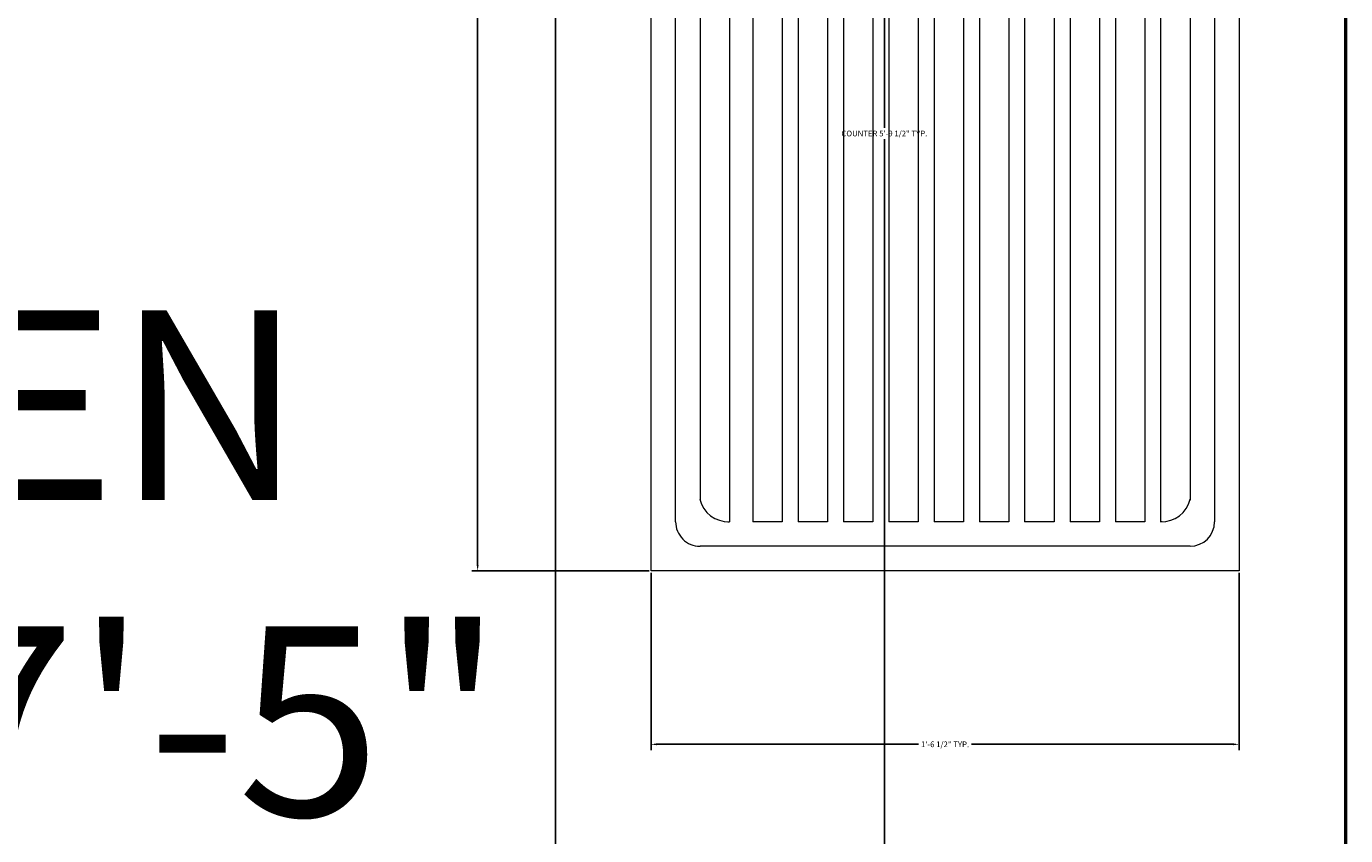
# Model space of a CAD drawing. Units: inches. Extents: x -173 to 545, y -746 to 104.
# Tile 27 of 32: x 219 to 261, y -69 to -43. Entities that reach past the tile are written whole.
import ezdxf

# ---------------------------------------------------------------- set-up
doc = ezdxf.new("R2010")
doc.units = ezdxf.units.IN
doc.header["$MEASUREMENT"] = 0
for name, color, linetype, lineweight in [('A-ANNO-DIMS', 2, 'Continuous', 18), ('A-AREA-IDEN', 7, 'Continuous', 18), ('A-FLOR-CASE', 9, 'Continuous', 25), ('A-FLOR-FIXT', 8, 'Continuous', 18), ('A-WALL', 7, 'Continuous', 50)]:
    doc.layers.add(name, color=color, linetype=linetype, lineweight=lineweight)
doc.styles.get("Standard").update_dxf_attribs({"font": 'arial.ttf'})
doc.dimstyles.get("Standard").update_dxf_attribs({"dimtxt": 0.18, "dimasz": 0.18, "dimexe": 0.18, "dimexo": 0.0625, "dimgap": 0.09, "dimtad": 0, "dimtih": 1, "dimtoh": 1, "dimdec": 0, "dimzin": 0, "dimdsep": 46, "dimlunit": 3, "dimtxsty": 'Standard', "dimcen": 0.09, "dimadec": 0, "dimazin": 0, "dimtfac": 1, "dimtdec": 0, "dimtofl": 0, "dimtmove": 0, "dimatfit": 3, "dimfxl": 1, "dimtolj": 1, "dimtzin": 0, "dimarcsym": 0})

# ---------------------------------------------------------------- blocks, each defined once
blk = doc.blocks.new('М11 540х1060')
for p, q in [((-1062, 540), (0, 540)), ((-1062, 0), (-1062, 540)), ((0, 540), (0, 0)), ((-1017, 517.5), (-45, 517.5)), ((-1039.5, 45), (-1039.5, 495)), ((-990, 495), (-589.5, 495)), ((-543.7, 495), (-64.8, 495)), ((-22.5, 495), (-22.5, 45)), ((-1017, 72), (-1017, 468)), ((-562.5, 72), (-562.5, 468)), ((-535.7, 468), (-45, 468)), ((-45, 469.5), (-45, 468)), ((-535.7, 453.4), (-45, 453.4)), ((-535.7, 453.4), (-535.7, 426.4)), ((-45, 453.4), (-45, 426.4)), ((-535.7, 426.4), (-45, 426.4)), ((-535.7, 411.8), (-535.7, 384.8)), ((-535.7, 411.8), (-45, 411.8)), ((-45, 411.8), (-45, 384.8)), ((-535.7, 384.8), (-45, 384.8)), ((-535.7, 370.1), (-535.7, 343.1)), ((-535.7, 370.1), (-45, 370.1)), ((-45, 370.1), (-45, 343.1)), ((-535.7, 343.1), (-45, 343.1)), ((-535.7, 328.5), (-535.7, 301.5)), ((-535.7, 328.5), (-45, 328.5)), ((-45, 328.5), (-45, 301.5)), ((-535.7, 301.5), (-45, 301.5)), ((-535.7, 286.9), (-535.7, 259.9)), ((-535.7, 286.9), (-45, 286.9)), ((-45, 286.9), (-45, 259.9)), ((-535.7, 259.9), (-45, 259.9)), ((-535.7, 245.3), (-535.7, 218.3)), ((-535.7, 245.3), (-45, 245.3)), ((-45, 245.3), (-45, 218.3)), ((-535.7, 218.3), (-45, 218.3)), ((-535.7, 203.6), (-535.7, 176.6)), ((-535.7, 203.6), (-45, 203.6)), ((-45, 203.6), (-45, 176.6)), ((-535.7, 176.6), (-45, 176.6)), ((-535.7, 162), (-45, 162)), ((-535.7, 162), (-535.7, 135)), ((-45, 162), (-45, 135)), ((-535.7, 135), (-45, 135)), ((-535.7, 120.4), (-45, 120.4)), ((-535.7, 120.4), (-535.7, 93.4)), ((-45, 120.4), (-45, 93.4)), ((-535.7, 93.4), (-45, 93.4)), ((-535.7, 72), (-45, 72)), ((-535.7, 72), (-535.7, 67.5)), ((-45, 70.5), (-45, 72)), ((-589.5, 45), (-990, 45)), ((-543.7, 45), (-64.8, 45)), ((-45, 22.5), (-1017, 22.5)), ((0, 0), (-1062, 0))]:
    blk.add_line(p, q)
for centre, major_axis, start_param, end_param in [((-1017, 495), (-15.9, 15.9), -0.785398, 0.785398), ((-45, 495), (15.9, 15.9), 5.497787, 7.068583), ((-990, 468), (19.1, 19.1), 0.785398, 2.356194), ((-589.5, 468), (-19.1, 19.1), 3.926991, 5.497787), ((-585.2, 468), (-35, 35), 3.926991, 4.503922), ((-72.3, 468.8), (-19.3, 19.3), 3.899365, 5.250385), ((-787.5, 270), (-19.1, 19.1), 3.926991, 10.210176), ((-787.5, 270), (-15.9, 15.9), 3.926991, 10.210176), ((-990, 72), (-19.1, 19.1), 0.785398, 2.356194), ((-589.5, 72), (19.1, 19.1), 3.926991, 5.497787), ((-585.2, 72), (35, 35), 4.920856, 5.497787), ((-72.3, 71.2), (19.3, 19.3), 4.174393, 5.525413), ((-1017, 45), (15.9, 15.9), 2.356194, 3.926991), ((-45, 45), (-15.9, 15.9), 2.356194, 3.926991)]:
    blk.add_ellipse(centre, major_axis=major_axis, ratio=1, start_param=start_param, end_param=end_param)
blk = doc.blocks.new('COUNTER-L-RETURN')
blk.add_line((66, 0), (66, 69.362))
blk = doc.blocks.new('*D42')
at = {"layer": 'A-ANNO-DIMS', "color": 0, "lineweight": -2, "transparency": 16777216}
for p, q in [((238.763, -23.923), (233.157, -23.923)), ((233.337, -24.103), (233.337, -42.033)), ((233.337, -60.33), (233.337, -42.4)), ((238.763, -60.51), (233.157, -60.51))]:
    blk.add_line(p, q, dxfattribs=at)
at = {"layer": 'A-ANNO-DIMS', "color": 0, "transparency": 16777216}
for points in [[(233.307, -24.103), (233.367, -24.103), (233.337, -23.923)], [(233.307, -60.33), (233.367, -60.33), (233.337, -60.51)]]:
    blk.add_solid(points, dxfattribs=at)
at = {"layer": 'Defpoints', "color": 0, "transparency": 16777216}
for p in [(238.825, -23.923), (233.337, -60.51), (238.825, -60.51)]:
    blk.add_point(p, dxfattribs=at)
at = {"layer": 'A-ANNO-DIMS', "color": 0, "transparency": 16777216, "insert": (233.337, -42.217), "char_height": 0.18, "attachment_point": 5}
blk.add_mtext('\\A1;SINK 3\'-0 1/2" TYP.', dxfattribs=at)
blk = doc.blocks.new('*D43')
at = {"layer": 'A-ANNO-DIMS', "color": 0, "lineweight": -2, "transparency": 16777216}
for p, q in [((238.825, -60.573), (238.825, -66.179)), ((257.429, -60.573), (257.429, -66.179)), ((239.005, -65.999), (247.288, -65.999)), ((257.249, -65.999), (248.967, -65.999))]:
    blk.add_line(p, q, dxfattribs=at)
at = {"layer": 'A-ANNO-DIMS', "color": 0, "transparency": 16777216}
for points in [[(239.005, -65.969), (239.005, -66.029), (238.825, -65.999)], [(257.249, -65.969), (257.249, -66.029), (257.429, -65.999)]]:
    blk.add_solid(points, dxfattribs=at)
at = {"layer": 'Defpoints', "color": 0, "transparency": 16777216}
for p in [(238.825, -60.51), (257.429, -60.51), (257.429, -65.999)]:
    blk.add_point(p, dxfattribs=at)
at = {"layer": 'A-ANNO-DIMS', "color": 0, "transparency": 16777216, "insert": (248.127, -65.999), "char_height": 0.18, "attachment_point": 5}
blk.add_mtext('\\A1;1\'-6 1/2" TYP.', dxfattribs=at)
blk = doc.blocks.new('*D76')
at = {"layer": 'A-ANNO-DIMS', "color": 0, "lineweight": -2, "transparency": 16777216}
for p, q in [((235.864, -12), (246.386, -12)), ((246.206, -12.18), (246.206, -46.498)), ((246.206, -81.182), (246.206, -46.864)), ((235.864, -81.362), (246.386, -81.362))]:
    blk.add_line(p, q, dxfattribs=at)
at = {"layer": 'A-ANNO-DIMS', "color": 0, "transparency": 16777216}
for points in [[(246.176, -12.18), (246.236, -12.18), (246.206, -12)], [(246.176, -81.182), (246.236, -81.182), (246.206, -81.362)]]:
    blk.add_solid(points, dxfattribs=at)
at = {"layer": 'Defpoints', "color": 0, "transparency": 16777216}
for p in [(235.801, -12), (246.206, -12), (235.801, -81.362)]:
    blk.add_point(p, dxfattribs=at)
at = {"layer": 'A-ANNO-DIMS', "color": 0, "transparency": 16777216, "insert": (246.206, -46.681), "char_height": 0.18, "attachment_point": 5}
blk.add_mtext('\\A1;COUNTER 5\'-9 1/2" TYP.', dxfattribs=at)

msp = doc.modelspace()

# ---------------------------------------------------------------- linework, layer by layer
at = {"layer": 'A-WALL'}
msp.add_line((260.801, 7.638), (260.801, -81.362), dxfattribs=at)

# ---------------------------------------------------------------- block references
at = {"layer": 'A-FLOR-CASE'}
msp.add_blockref('COUNTER-L-RETURN', (169.801, -81.362), dxfattribs=at)
at = {"layer": 'A-FLOR-FIXT', "xscale": 0.0344518369672997, "yscale": 0.0344518369672997, "zscale": 0.0344518369672997, "rotation": 270}
msp.add_blockref('М11 540х1060', (238.825, -60.51), dxfattribs=at)

# ---------------------------------------------------------------- texts
at = {"layer": 'A-AREA-IDEN', "insert": (193.303, -52.27), "char_height": 6, "attachment_point": 1}
msp.add_mtext('KITCHEN\\P7\'-7"X7\'-5"', dxfattribs=at)

# ---------------------------------------------------------------- dimensions: what is measured, and where the dimension line sits
at = {"layer": 'A-ANNO-DIMS'}
for base, p1, p2, angle, text, picture, middle in [((246.206, -12), (235.801, -81.362), (235.801, -12), 90, 'COUNTER <> TYP.', '*D76', (246.206, -46.681)), ((233.337, -60.51), (238.825, -23.923), (238.825, -60.51), 270, 'SINK <> TYP.', '*D42', (233.337, -42.217))]:
    dim = msp.add_linear_dim(base=base, p1=p1, p2=p2, angle=angle, text=text, dimstyle='Standard', override={"dimdec": 1, "dimlfac": 1, "dimrnd": 0, "dimzin": 1, "dimdsep": 46, "dimlunit": 4, "dimfrac": 2}, dxfattribs=at)
    dim.commit()
    dim.dimension.update_dxf_attribs({"geometry": picture, "text_midpoint": middle})
dim = msp.add_linear_dim(base=(257.429, -65.999), p1=(238.825, -60.51), p2=(257.429, -60.51), text='<> TYP.', dimstyle='Standard', override={"dimdec": 1, "dimlfac": 1, "dimrnd": 0, "dimzin": 1, "dimdsep": 46, "dimlunit": 4, "dimfrac": 2}, dxfattribs=at)
dim.commit()
dim.dimension.update_dxf_attribs({"geometry": '*D43', "text_midpoint": (248.127, -65.999)})

doc.saveas('drawing.dxf')
